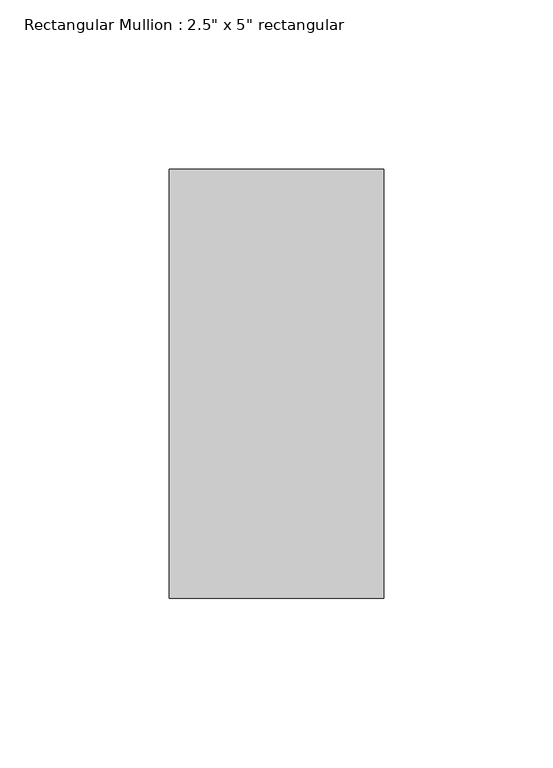
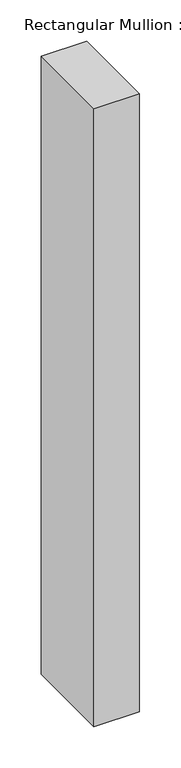
"""IFC4 building model written with IfcOpenShell, lengths in millimetres: member geometry."""

from ifc_helpers import new_model, si_unit, frame, origin, place, context, project, spatial, polyline, outline, extrude, source, transform, mapped, element, save


def member_8c3e4394(model_context):
    return source(origin(), model_context, "Body", "SweptSolid", [
        extrude(outline(polyline([(0.0, 63.5), (0.0, -63.5), (-63.5, -63.5), (-63.5, 63.5), (0.0, 63.5)])), frame((0.0, 0.0, -911.225), z_axis=(0.0, 0.0, 1.0), x_axis=(1.0, 0.0, 0.0)), (0.0, 0.0, 1.0), 911.225),
    ])


if __name__ == "__main__":
    model = new_model("IFC4")
    model_context = context("Model", 3, world=origin())
    ifc_project = project(units=[si_unit("LENGTHUNIT", "METRE", prefix="MILLI")], contexts=[model_context])
    site = spatial("IfcSite", under=ifc_project)
    building = spatial("IfcBuilding", under=site)
    placement = place(None, origin())
    member_shape = member_8c3e4394(model_context)
    element("IfcMember", 1, ObjectType="Rectangular Mullion : 2.5\" x 5\" rectangular", at=placement, inside=building, context=model_context, shape_type="MappedRepresentation", body=[
        mapped(member_shape, transform((0.0, 0.0, 0.0), x_axis=(1.0, 0.0, 0.0), y_axis=(0.0, 1.0, 0.0), z_axis=(0.0, 0.0, 1.0))),
    ])
    save(model, "model.ifc")

# Revit data of these elements
# Type "Rectangular Mullion : 2.5\" x 5\" rectangular"
#   built-in parameter 1007304 = 0.416667 (stored number, unit not read)
#   built-in parameter 1007301 = 0.104167 (stored number, unit not read)
#   built-in parameter 1007300 = 0.104167 (stored number, unit not read)
# Element 1 (IfcMember, "Rectangular Mullion : 2.5\" x 5\" rectangular")
#   Materials on its faces: "Aluminum"
# Materials
#   "Aluminum": class "Metal", colour RGB 247 247 247, transparency 0, Description = "Aluminum 6061", Cost = 0
